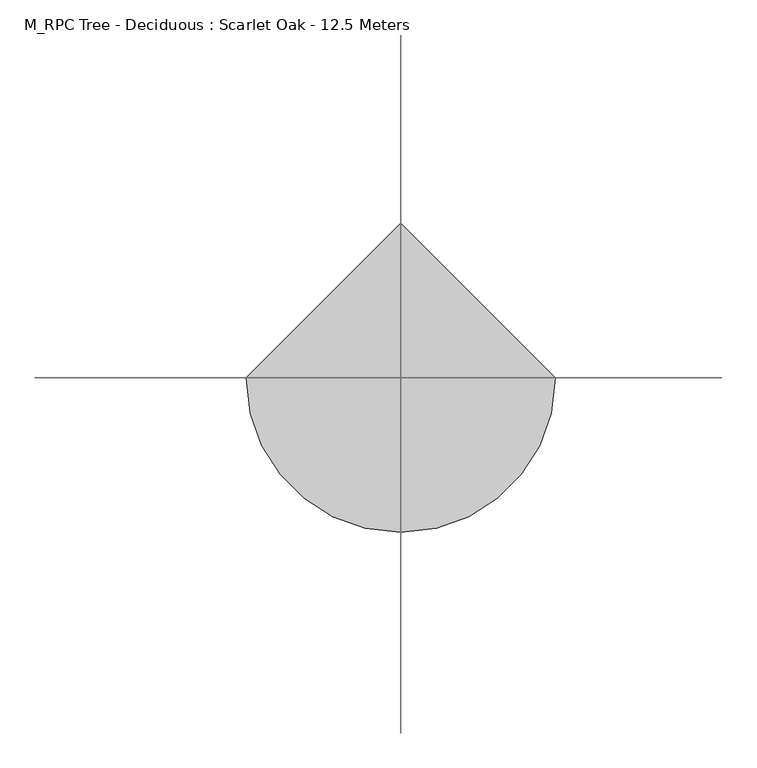
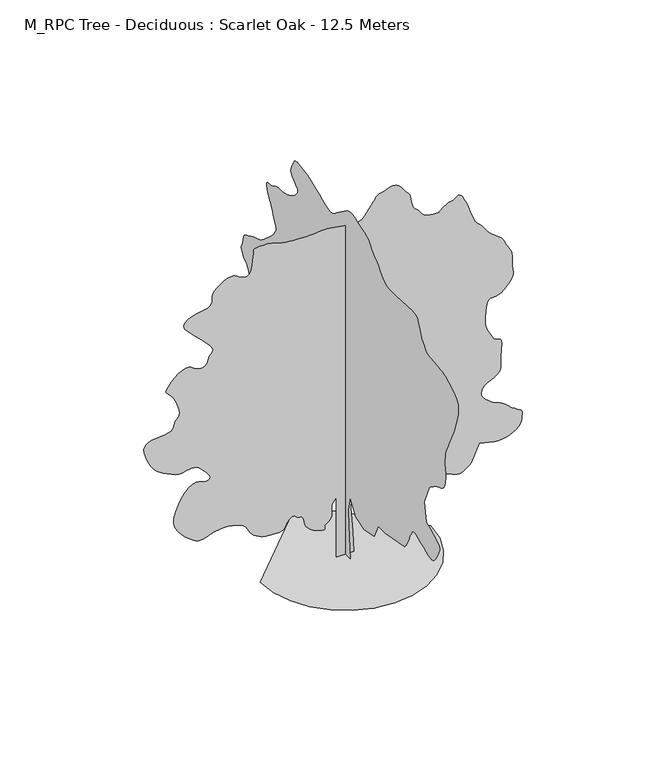
"""IFC4 building model written with IfcOpenShell, lengths in millimetres: geographic element geometry, M_RPC Tree - Deciduous : Scarlet Oak - 12.5 Meters."""

from ifc_helpers import new_model, si_unit, origin, place, context, project, spatial, triangles, source, transform, mapped, element, save


def m_rpc_tree_deciduous_scarlet_oak_12_5_meters_78a4568a(model_context):
    return source(origin(), model_context, "Body", "Tessellation", [
        triangles([(0.0172504, 306.0074844, 0.0), (0.0172504, -293.5650026, 0.0), (0.0172504, -196.8600042, 1141.1200275), (0.0172504, -177.5185068, 1682.6674953), (0.0172504, -293.5650026, 2185.5350567), (0.0172504, -603.0224945, 1682.6674953), (0.0172504, -1105.8875124, 1527.9400211), (0.0172504, -1686.1174301, 1663.3275421), (0.0172504, -1918.2099495, 2146.8525341), (0.0172504, -2324.3725124, 2146.8525341), (0.0172504, -3446.150116, 2359.6049549), (0.0172504, -3487.4249222, 2409.394939), (0.0172504, -3527.7000801, 2459.5225479), (0.0172504, -3565.9250725, 2510.3249702), (0.0172504, -3601.0999603, 2562.1500046), (0.0172504, -3632.2250954, 2615.3249565), (0.0172504, -3658.2749588, 2670.2000954), (0.0172504, -3678.2499023, 2727.0751122), (0.0172504, -3697.649881, 2785.6750237), (0.0172504, -3722.1251312, 2845.2748741), (0.0172504, -3750.8251236, 2905.7249634), (0.0172504, -3782.89991, 2966.8500114), (0.0172504, -3817.5251221, 3028.475029), (0.0172504, -3853.8249413, 3090.4500252), (0.0172504, -3890.9999977, 3152.5750122), (0.0172504, -3908.7000801, 3172.6499496), (0.0172504, -3933.1750397, 3188.8501236), (0.0172504, -3971.1750458, 3197.2499016), (0.0172504, -4029.4749756, 3193.9751015), (0.0172504, -4114.8499969, 3175.1500877), (0.0172504, -4234.0499886, 3136.8500999), (0.0172504, -4393.8501183, 3075.2250824), (0.0172504, -4562.5749939, 3002.6998581), (0.0172504, -4706.2499451, 2937.9750298), (0.0172504, -4828.2750549, 2886.4249786), (0.0172504, -4932.0251175, 2853.4999535), (0.0172504, -5020.8999252, 2844.5999153), (0.0172504, -5098.249855, 2865.125116), (0.0172504, -5167.5002792, 2920.4999336), (0.0172504, -5237.3750839, 3007.7251328), (0.0172504, -5309.5997452, 3113.9000473), (0.0172504, -5377.1002762, 3229.5499649), (0.0172504, -5432.7497864, 3345.1998825), (0.0172504, -5469.4498718, 3451.3750877), (0.0172504, -5480.1248016, 3538.6249947), (0.0172504, -5457.6250122, 3597.424894), (0.0172504, -5402.6498795, 3641.7000984), (0.0172504, -5323.3000717, 3691.0249947), (0.0172504, -5223.6747574, 3744.5999222), (0.0172504, -5107.774855, 3801.5499344), (0.0172504, -4979.7251129, 3861.0500816), (0.0172504, -4843.5499947, 3922.2251266), (0.0172504, -4703.3251236, 3984.2501198), (0.0172504, -4587.2749397, 4641.8500969), (0.0172504, -4877.3749649, 5318.7747665), (0.0172504, -4886.5249878, 5331.7001404), (0.0172504, -4900.7252838, 5347.4747589), (0.0172504, -4925.0999588, 5369.0251877), (0.0172504, -4964.6748688, 5399.20009), (0.0172504, -5024.5502838, 5440.8498734), (0.0172504, -5109.8247299, 5496.8999405), (0.0172504, -5225.5252258, 5570.225116), (0.0172504, -5351.0501221, 5636.6501312), (0.0172504, -5462.3497238, 5680.0498077), (0.0172504, -5559.4501923, 5715.3499786), (0.0172504, -5642.3497833, 5757.424736), (0.0172504, -5711.0252426, 5821.1499161), (0.0172504, -5765.4998245, 5921.4001923), (0.0172504, -5805.7502747, 6073.0752365), (0.0172504, -5829.0500153, 6222.0498642), (0.0172504, -5835.7501877, 6317.5748474), (0.0172504, -5830.6249191, 6379.6001312), (0.0172504, -5818.3750854, 6428.1000778), (0.0172504, -5803.7748138, 6483.0252136), (0.0172504, -5791.5499786, 6564.3249023), (0.0172504, -5786.4247101, 6692.0002487), (0.0172504, -5788.2251816, 6832.849791), (0.0172504, -5796.1252808, 6949.6752182), (0.0172504, -5813.8247818, 7056.3751007), (0.0172504, -5845.0502014, 7166.7747574), (0.0172504, -5893.550148, 7294.7750839), (0.0172504, -5963.0249771, 7454.2502335), (0.0172504, -6057.1750443, 7659.049942), (0.0172504, -6146.5748199, 7844.1752701), (0.0172504, -6206.1752518, 7955.8748474), (0.0172504, -6246.4751175, 8024.9502823), (0.0172504, -6277.9999374, 8082.1752777), (0.0172504, -6311.225235, 8158.3502792), (0.0172504, -6356.599791, 8284.2751511), (0.0172504, -6424.6752869, 8490.6997604), (0.0172504, -6498.0248795, 8729.4997192), (0.0172504, -6547.3747742, 8935.1499573), (0.0172504, -6565.2498459, 9112.3751862), (0.0172504, -6544.199968, 9265.925116), (0.0172504, -6476.8250107, 9400.5250397), (0.0172504, -6355.6498489, 9520.9002502), (0.0172504, -6173.2249374, 9631.8248749), (0.0172504, -5996.2252762, 9723.0001236), (0.0172504, -5879.7998245, 9785.7747803), (0.0172504, -5799.2250916, 9827.2001587), (0.0172504, -5729.8002594, 9854.4496582), (0.0172504, -5646.85009, 9874.575174), (0.0172504, -5525.6749283, 9894.699527), (0.0172504, -5341.575119, 9921.9501892), (0.0172504, -5144.0999634, 9943.4244598), (0.0172504, -4990.9500092, 9951.725116), (0.0172504, -4869.5998581, 9962.0244873), (0.0172504, -4767.5499825, 9989.5995483), (0.0172504, -4672.2499855, 10049.6505341), (0.0172504, -4571.2000488, 10157.425351), (0.0172504, -4451.8750648, 10328.0998169), (0.0172504, -4347.6750298, 10515.7499908), (0.0172504, -4286.1000092, 10666.5500885), (0.0172504, -4245.8501404, 10783.8254883), (0.0172504, -4205.5749825, 10871.0003998), (0.0172504, -4143.9999619, 10931.4501984), (0.0172504, -4039.7999268, 10968.5502594), (0.0172504, -3871.650016, 10985.7003754), (0.0172504, -2943.2749969, 10927.6748474), (0.0172504, -2772.1499771, 10930.6746643), (0.0172504, -2632.8250511, 10930.2746887), (0.0172504, -2514.4500092, 10937.3254211), (0.0172504, -2406.244986, 10962.6250397), (0.0172504, -2297.3600624, 11017.0496246), (0.0172504, -2176.9724979, 11111.3752625), (0.0172504, -2034.2550465, 11256.4745453), (0.0172504, -1896.7275398, 11403.0249023), (0.0172504, -1793.7050491, 11502.8746216), (0.0172504, -1717.0749882, 11568.5752625), (0.0172504, -1658.7125622, 11612.6248993), (0.0172504, -1610.5025688, 11647.5250946), (0.0172504, -1564.320068, 11685.7995026), (0.0172504, -1512.0500027, 11739.9996826), (0.0172504, -1461.8649845, 11804.0004272), (0.0172504, -1420.8125484, 11863.6002777), (0.0172504, -1379.087479, 11919.1503754), (0.0172504, -1326.8724976, 11970.9495392), (0.0172504, -1254.3574471, 12019.4000702), (0.0172504, -1151.7299904, 12064.7996246), (0.0172504, -1009.182514, 12107.4749268), (0.0172504, -849.1549999, 12154.4999634), (0.0172504, -699.9524792, 12206.6002716), (0.0172504, -560.5600064, 12254.6496643), (0.0172504, -429.9675053, 12289.4998627), (0.0172504, -307.1550161, 12302.0246796), (0.0172504, -191.1079934, 12283.0746735), (0.0172504, -80.8134993, 12223.5248199), (0.0172504, 499.4175176, 11798.0252106), (0.0172504, 562.2325061, 11740.8496307), (0.0172504, 623.0199657, 11688.7504852), (0.0172504, 689.217524, 11646.7751404), (0.0172504, 768.2749804, 11620.0500275), (0.0172504, 867.630035, 11613.6248383), (0.0172504, 994.7275097, 11632.5748444), (0.0172504, 1157.0125168, 11681.9753174), (0.0172504, 1341.1749676, 11755.3254913), (0.0172504, 1526.6899521, 11837.8251068), (0.0172504, 1710.1749733, 11922.0246185), (0.0172504, 1888.2475342, 12000.4500641), (0.0172504, 2057.5249924, 12065.6995697), (0.0172504, 2214.6200546, 12110.3003357), (0.0172504, 2356.1550201, 12126.8249084), (0.0172504, 2484.8875694, 12135.849939), (0.0172504, 2604.4750374, 12156.3754303), (0.0172504, 2712.9251038, 12178.575238), (0.0172504, 2808.1501053, 12192.6755402), (0.0172504, 2888.1748718, 12188.8501923), (0.0172504, 2950.9251114, 12157.2753754), (0.0172504, 2994.400074, 12088.1249451), (0.0172504, 3033.2500282, 12001.2500153), (0.0172504, 3077.8499222, 11921.1246735), (0.0172504, 3119.7499809, 11845.0502472), (0.0172504, 3150.5001389, 11770.3245758), (0.0172504, 3161.6000427, 11694.2745667), (0.0172504, 3144.6249161, 11614.1503876), (0.0172504, 3091.124984, 11527.2498779), (0.0172504, 3009.2500397, 11447.6245056), (0.0172504, 2921.5998665, 11385.2504059), (0.0172504, 2841.4251091, 11331.3502075), (0.0172504, 2781.8749649, 11277.1000305), (0.0172504, 2756.1750801, 11213.7248291), (0.0172504, 2777.4749428, 11132.4251404), (0.0172504, 2859.0249069, 11024.3747589), (0.0172504, 2971.6250107, 10916.7255157), (0.0172504, 3077.7999252, 10838.2000763), (0.0172504, 3178.2249001, 10782.3), (0.0172504, 3273.574894, 10742.6745117), (0.0172504, 3364.5248657, 10712.8251709), (0.0172504, 3451.7750633, 10686.4000397), (0.0172504, 3535.9498672, 10656.8995148), (0.0172504, 3620.024968, 10634.1753204), (0.0172504, 3706.4749237, 10626.6746155), (0.0172504, 3795.2750267, 10625.9502411), (0.0172504, 3886.4499847, 10623.5248077), (0.0172504, 3980.0000885, 10610.9499939), (0.0172504, 4075.9250473, 10579.7495728), (0.0172504, 4174.1998627, 10521.5252197), (0.0172504, 4275.775058, 10469.80047), (0.0172504, 4375.6250679, 10451.2504395), (0.0172504, 4465.0001358, 10446.8995422), (0.0172504, 4535.0999268, 10437.8245148), (0.0172504, 4577.0999794, 10405.075351), (0.0172504, 4582.2249573, 10329.6753021), (0.0172504, 4541.7001053, 10192.7255219), (0.0172504, 4481.7999825, 10048.5994354), (0.0172504, 4432.0751106, 9951.4995483), (0.0172504, 4388.424868, 9882.1247131), (0.0172504, 4346.8250816, 9821.224942), (0.0172504, 4303.1751297, 9749.5002502), (0.0172504, 4253.4249687, 9647.6750702), (0.0172504, 4193.550135, 9496.4499985), (0.0172504, 4130.2749275, 9347.6997757), (0.0172504, 4075.8250534, 9253.7502777), (0.0172504, 4034.1999779, 9195.999733), (0.0172504, 4009.500032, 9155.8498581), (0.0172504, 4005.7749687, 9114.7000443), (0.0172504, 4027.1001205, 9053.900267), (0.0172504, 4077.4999512, 8954.8999146), (0.0172504, 4167.2249977, 8823.6747849), (0.0172504, 4293.1248711, 8684.3501495), (0.0172504, 4439.3499573, 8545.349913), (0.0172504, 4589.9500671, 8415.1497208), (0.0172504, 4729.0750053, 8302.2002197), (0.0172504, 4840.7748734, 8214.9747299), (0.0172504, 4909.1747681, 8161.9000626), (0.0172504, 4969.9001312, 8128.6997635), (0.0172504, 5061.0747986, 8095.1500671), (0.0172504, 5170.5250946, 8060.9248306), (0.0172504, 5286.0750183, 8025.675238), (0.0172504, 5395.524733, 7989.0751465), (0.0172504, 5486.6999817, 7950.8001572), (0.0172504, 5547.4247635, 7910.4747116), (0.0172504, 5598.275148, 7876.9750122), (0.0172504, 5663.0252655, 7853.2997131), (0.0172504, 5734.1749924, 7830.2999542), (0.0172504, 5804.3247803, 7798.8251312), (0.0172504, 5866.0250839, 7749.7752182), (0.0172504, 5911.8001968, 7673.9751938), (0.0172504, 5934.2499893, 7562.325032), (0.0172504, 5952.6250305, 7450.1749008), (0.0172504, 5984.1998474, 7370.8500916), (0.0172504, 6018.4750809, 7312.1501862), (0.0172504, 6045.000206, 7261.899765), (0.0172504, 6053.2252853, 7207.9501511), (0.0172504, 6032.699794, 7138.074765), (0.0172504, 5972.9249542, 7040.1249298), (0.0172504, 5898.7248322, 6948.3747162), (0.0172504, 5838.7250061, 6893.5251572), (0.0172504, 5788.2001831, 6857.9500031), (0.0172504, 5742.4000717, 6824.0497467), (0.0172504, 5696.6249588, 6774.2498795), (0.0172504, 5646.1001358, 6690.9747299), (0.0172504, 5586.0997284, 6556.5997925), (0.0172504, 5520.7002319, 6421.9998688), (0.0172504, 5460.6998245, 6337.1498154), (0.0172504, 5411.5249191, 6283.075209), (0.0172504, 5378.6001846, 6240.824881), (0.0172504, 5367.3247101, 6191.4999847), (0.0172504, 5383.09991, 6116.0999359), (0.0172504, 5431.3748703, 5995.7247253), (0.0172504, 5495.5000259, 5864.0502045), (0.0172504, 5555.8748291, 5761.8250488), (0.0172504, 5613.5747955, 5680.5747757), (0.0172504, 5669.5498672, 5611.8249023), (0.0172504, 5724.8749786, 5547.1497803), (0.0172504, 5780.5250702, 5478.0749268), (0.0172504, 5837.5250793, 5396.1502762), (0.0172504, 5903.6751114, 5315.3499756), (0.0172504, 5980.6500641, 5249.4249298), (0.0172504, 6060.324852, 5189.6000931), (0.0172504, 6134.5999695, 5127.0498413), (0.0172504, 6195.3247513, 5053.0252899), (0.0172504, 6234.4002731, 4958.675235), (0.0172504, 6243.7002869, 4835.2499199), (0.0172504, 6251.5248093, 4738.3250221), (0.0172504, 6280.349794, 4706.349939), (0.0172504, 6313.2251129, 4704.825032), (0.0172504, 6333.2500534, 4699.2500816), (0.0172504, 6323.4750687, 4655.0998695), (0.0172504, 6267.0500244, 4537.8750481), (0.0172504, 6146.999794, 4313.0501083), (0.0172504, 6021.4748978, 4060.8750938), (0.0172504, 5945.6998718, 3875.3750793), (0.0172504, 5898.3248566, 3742.6250427), (0.0172504, 5858.0749878, 3648.7999557), (0.0172504, 5803.5998245, 3580.0000854), (0.0172504, 5713.6000854, 3522.3751144), (0.0172504, 5566.7747452, 3462.0500175), (0.0172504, 5397.250209, 3413.1000984), (0.0172504, 5248.0500137, 3392.5748978), (0.0172504, 5111.025238, 3390.9999939), (0.0172504, 4978.0752136, 3398.9000931), (0.0172504, 4841.0498566, 3406.7749031), (0.0172504, 4691.8499519, 3405.1999992), (0.0172504, 4522.3501236, 3384.6750893), (0.0172504, 4353.2999771, 3366.3000481), (0.0172504, 4207.2498802, 3370.2500977), (0.0172504, 4078.7998718, 3385.7000267), (0.0172504, 3962.5249924, 3401.8249146), (0.0172504, 3853.0249901, 3407.8001312), (0.0172504, 3744.8749054, 3392.799884), (0.0172504, 3632.6500694, 3346.0001244), (0.0172504, 3525.249939, 3296.2499634), (0.0172504, 3436.4251282, 3270.2000999), (0.0172504, 3368.249929, 3253.6249489), (0.0172504, 3322.75009, 3232.3250862), (0.0172504, 3301.9499062, 3192.0499283), (0.0172504, 3307.8751259, 3118.6500481), (0.0172504, 3342.5500443, 2997.8498634), (0.0172504, 3398.475119, 2869.5251381), (0.0172504, 3465.5750931, 2778.7248665), (0.0172504, 3542.0000793, 2719.2500084), (0.0172504, 3625.8499031, 2684.8000763), (0.0172504, 3715.274968, 2669.1248703), (0.0172504, 3808.4250961, 2665.9500641), (0.0172504, 3903.4251114, 2669.0498749), (0.0172504, 4270.9250633, 2262.8999565), (0.0172504, 4299.7250496, 2217.1674282), (0.0172504, 4327.3501076, 2170.5925095), (0.0172504, 4352.6250183, 2122.3249615), (0.0172504, 4374.3248566, 2071.5174522), (0.0172504, 4391.2999832, 2017.3300621), (0.0172504, 4402.3498901, 1958.9125523), (0.0172504, 4406.2999397, 1895.4200615), (0.0172504, 4405.6249809, 1829.2200325), (0.0172504, 4400.8999786, 1763.6974331), (0.0172504, 4388.0248924, 1699.5299835), (0.0172504, 4362.9999664, 1637.3900265), (0.0172504, 4321.7248695, 1577.9574623), (0.0172504, 4260.1501396, 1521.9075405), (0.0172504, 4174.1998627, 1469.9175453), (0.0172504, 4092.2249245, 1425.7650078), (0.0172504, 4034.5999535, 1391.4249527), (0.0172504, 3985.4250481, 1364.8675621), (0.0172504, 3928.800016, 1344.0599659), (0.0172504, 3848.8499542, 1326.9749622), (0.0172504, 3729.6499626, 1311.5799717), (0.0172504, 3555.3001396, 1295.8475018), (0.0172504, 3356.9750359, 1298.1024513), (0.0172504, 3174.2251442, 1332.8375404), (0.0172504, 3003.6500908, 1392.27243), (0.0172504, 2841.8750816, 1468.6199501), (0.0172504, 2685.525032, 1554.1049938), (0.0172504, 2531.1748604, 1640.9425713), (0.0172504, 2375.4949734, 1721.3500179), (0.0172504, 2236.6675461, 1794.4849434), (0.0172504, 2129.3050587, 1863.5599422), (0.0172504, 2044.6099377, 1926.8850014), (0.0172504, 1973.7875164, 1982.7650208), (0.0172504, 1908.0399307, 2029.5099873), (0.0172504, 1838.5700432, 2065.4300331), (0.0172504, 1756.5824604, 2088.8300583), (0.0172504, 1666.4174698, 2108.5650455), (0.0172504, 1577.6074837, 2133.0375343), (0.0172504, 1489.134977, 2159.8799366), (0.0172504, 1399.9875114, 2186.7200134), (0.0172504, 1309.1449459, 2211.1925022), (0.0172504, 1215.5975309, 2230.9274895), (0.0172504, 1118.3299942, 2243.5575325), (0.0172504, 1018.8625191, 2250.1549496), (0.0172504, 919.3925005, 2253.7074944), (0.0172504, 819.9250254, 2254.7225487), (0.0172504, 720.4574776, 2253.7074944), (0.0172504, 620.9900024, 2251.1700039), (0.0172504, 521.5199839, 2247.6174591), (0.0172504, 422.0525087, 2243.5575325), (0.0172504, 228.6430025, 1953.4425373), (0.0172504, 189.960498, 1508.6000679), (280.4450004, 0.0006008, 0.0092122), (-299.7850081, 0.0006008, 0.0092122), (-299.7850081, 0.0004756, 2127.5199932), (-454.5149895, 0.0004756, 1914.7700432), (-454.5149895, 0.0005007, 1682.6775238), (-450.9625174, 0.0005007, 1628.8274677), (-450.9625174, 0.0005007, 1575.1449886), (-458.0674979, 0.0005007, 1521.8024597), (-475.8274967, 0.0005257, 1468.967458), (-507.8000001, 0.0005257, 1416.8100311), (-557.5350094, 0.0005257, 1365.4949947), (-628.5824896, 0.0005257, 1315.1974834), (-684.2375227, 0.0005257, 1262.982502), (-699.6325132, 0.0005257, 1210.0900183), (-696.0799685, 0.0005257, 1162.9524885), (-694.8950117, 0.0005257, 1127.990015), (-717.3950191, 0.0005257, 1111.6375248), (-784.8900272, 0.0005257, 1120.3225325), (-918.6974848, 0.0005257, 1160.4700092), (-1071.3399845, 0.0005257, 1223.0050003), (-1185.4125275, 0.0005257, 1293.6575191), (-1267.3425556, 0.0005257, 1371.0799736), (-1323.5625252, 0.0005257, 1453.9125629), (-1360.49748, 0.0005007, 1540.8049335), (-1384.5749348, 0.0005007, 1630.4049877), (-1402.2250202, 0.0005007, 1721.3600464), (-1406.7350647, 0.0005007, 1746.1124599), (-1413.4449749, 0.0005007, 1770.19006), (-1424.5524364, 0.0005007, 1792.9174519), (-1442.2599312, 0.0005007, 1813.6099388), (-1468.7600578, 0.0005007, 1831.5975037), (-1506.2599491, 0.0005007, 1846.2025715), (-1556.9524944, 0.0005007, 1856.7475674), (-1607.6450397, 0.0005007, 1874.1124958), (-1647.5100483, 0.0005007, 1903.3224861), (-1682.3025467, 0.0004756, 1934.9000645), (-1717.7700039, 0.0004756, 1959.3725533), (-1759.6674465, 0.0004756, 1967.2675655), (-1813.7424889, 0.0004756, 1949.1099529), (-1885.7500122, 0.0005007, 1895.4274738), (-1949.0724552, 0.0005007, 1820.3199944), (-1984.9925011, 0.0005007, 1746.902528), (-2011.1000645, 0.0005007, 1679.2374722), (-2044.9875309, 0.0005007, 1621.382428), (-2104.2525181, 0.0005007, 1577.4025543), (-2206.4824699, 0.0005007, 1551.3499294), (-2369.2750042, 0.0005007, 1547.2900028), (-2549.149926, 0.0005007, 1559.2449417), (-2695.2000229, 0.0005007, 1578.979929), (-2813.8250496, 0.0005007, 1607.1750103), (-2911.4999016, 0.0005007, 1644.5025284), (-2994.6250603, 0.0005007, 1691.6425289), (-3069.600135, 0.0005007, 1749.2724415), (-3142.9250198, 0.0005007, 1818.0650448), (-3205.1000038, 0.0005007, 1893.5100037), (-3249.7248962, 0.0004756, 1969.2975288), (-3287.549913, 0.0004756, 2043.389954), (-3329.4499718, 0.0004756, 2113.7625481), (-3386.2249947, 0.0004756, 2178.3824409), (-3468.7249008, 0.0004756, 2235.2224308), (-3587.7499031, 0.0004756, 2282.2499382), (-3707.4248657, 0.0004756, 2317.9974655), (-3794.2500893, 0.0004506, 2343.2600224), (-3862.8249733, 0.0004506, 2359.3875263), (-3927.6750847, 0.0004506, 2367.7325111), (-4003.3251183, 0.0004506, 2369.6499813), (-4104.3750549, 0.0004506, 2366.4924706), (-4245.3498802, 0.0004506, 2359.6125126), (-4400.3500122, 0.0004506, 2335.1974331), (-4538.1250328, 0.0004756, 2289.8050003), (-4665.0501343, 0.0004756, 2240.3524956), (-4787.5749229, 0.0004756, 2203.7574909), (-4912.1501678, 0.0004756, 2196.9349422), (-5045.1501892, 0.0004756, 2236.7999508), (-5193.0498825, 0.0004506, 2340.2725594), (-5347.7997391, 0.0004506, 2478.6475433), (-5490.6747391, 0.0004506, 2615.9999153), (-5612.2498764, 0.0004256, 2758.4499413), (-5703.0251495, 0.0004256, 2912.049868), (-5753.5499725, 0.0004256, 3082.8999046), (-5754.3499237, 0.0004005, 3277.0999695), (-5695.9250015, 0.0004005, 3500.7249825), (-5598.1501556, 0.0003755, 3726.2748779), (-5489.1998291, 0.0003755, 3919.6999901), (-5372.1499969, 0.0003505, 4077.2499664), (-5250.0248932, 0.0003505, 4195.2000343), (-5125.8499146, 0.0003505, 4269.8501289), (-5002.6998734, 0.0003505, 4297.4998947), (-4883.6001663, 0.0003505, 4274.3751434), (-4771.2750458, 0.0003505, 4235.4749016), (-4671.8250114, 0.0003505, 4218.8750427), (-4593.3248611, 0.0003505, 4225.6499199), (-4543.9249695, 0.0003505, 4256.7750549), (-4531.7501312, 0.0003505, 4313.2750946), (-4564.9001427, 0.0003505, 4396.1749763), (-4651.5000893, 0.0003254, 4506.4749298), (-4752.500029, 0.0003254, 4617.0998634), (-4829.4749817, 0.0003254, 4702.3498924), (-4891.5502625, 0.0003254, 4765.2751213), (-4947.8747314, 0.0003254, 4808.9250732), (-5007.6001556, 0.0003254, 4836.325145), (-5079.8248169, 0.0003004, 4850.5498581), (-5173.7248993, 0.0003004, 4854.5999016), (-5270.0248352, 0.0003254, 4845.5248741), (-5349.7751999, 0.0003254, 4824.5999886), (-5422.3998367, 0.0003254, 4801.3249557), (-5497.39991, 0.0003254, 4785.1250725), (-5584.2248428, 0.0003254, 4785.5250481), (-5692.3752182, 0.0003254, 4811.9748871), (-5831.3248764, 0.0003004, 4873.9498833), (-5978.7751785, 0.0003004, 4948.0997177), (-6108.6248108, 0.0003004, 5012.4248611), (-6224.6252884, 0.0003004, 5078.4748993), (-6330.4502243, 0.0003004, 5157.6997147), (-6429.8749695, 0.0003004, 5261.5997681), (-6526.574881, 0.0002754, 5401.7249359), (-6624.2997299, 0.0002754, 5589.5750977), (-6705.1000305, 0.0002503, 5784.4998276), (-6749.7002151, 0.0002503, 5941.2001465), (-6759.8001801, 0.0002503, 6064.0752045), (-6737.074823, 0.0002253, 6157.4997345), (-6683.2252029, 0.0002253, 6225.9002106), (-6599.9500534, 0.0002253, 6273.6502029), (-6488.899855, 0.0002253, 6305.1750229), (-6357.7997177, 0.0002253, 6323.2750809), (-6219.2750336, 0.0002253, 6333.9500107), (-6082.4002487, 0.0002253, 6346.2748398), (-5956.3748016, 0.0002253, 6369.4501694), (-5850.3248795, 0.0002253, 6412.5998611), (-5773.3499268, 0.0002253, 6484.8251038), (-5734.5999664, 0.0002003, 6595.2997559), (-5705.9749695, 0.0002003, 6701.9752213), (-5661.749762, 0.0002003, 6771.4500504), (-5614.8497177, 0.0002003, 6825.7002274), (-5578.0752182, 0.0002003, 6886.6999924), (-5564.3248947, 0.0001752, 6976.4747452), (-5586.4252899, 0.0001752, 7116.9998886), (-5657.2500366, 0.0001752, 7330.2502441), (-5757.5497284, 0.0001502, 7540.3002136), (-5853.4752686, 0.0001502, 7672.5252823), (-5935.8498917, 0.0001502, 7750.975145), (-5995.5747345, 0.0001252, 7799.6250824), (-6023.4747757, 0.0001252, 7842.5247894), (-6010.4499893, 0.0001252, 7903.7251236), (-5947.3497711, 0.0001252, 8007.2002029), (-5845.6501648, 0.0001252, 8136.3248795), (-5728.0247864, 0.0001001, 8253.9502579), (-5602.2749039, 0.0001001, 8353.3000076), (-5476.1750427, 0.0001001, 8427.6251221), (-5357.5497253, 0.0001001, 8470.1248535), (-5254.1252243, 0.0001001, 8474.0751938), (-5173.7248993, 0.0001001, 8432.6998123), (-5094.9000595, 0.0001001, 8371.00009), (-4997.8001724, 0.0001001, 8322.8501221), (-4892.5751999, 0.0001001, 8294.6500992), (-4789.3751038, 0.0001001, 8292.850209), (-4698.375135, 0.0001001, 8323.8750595), (-4629.6999664, 0.0001001, 8394.1248413), (-4593.5001411, 0.0001001, 8510.0497421), (-4560.3251312, 0.0001001, 8620.5749725), (-4508.2251137, 7.51e-05, 8686.1000427), (-4458.4999512, 7.51e-05, 8730.3002518), (-4432.4500877, 7.51e-05, 8776.8747345), (-4451.4000938, 7.51e-05, 8849.4999527), (-4536.6501228, 7.51e-05, 8971.8750412), (-4709.5500343, 5.01e-05, 9167.6497192), (-4926.3498825, 5.01e-05, 9388.800174), (-5120.1502625, 2.5e-05, 9575.0998489), (-5277.4249649, 2.5e-05, 9731.9751572), (-5384.5998184, 2.5e-05, 9864.8246063), (-5428.2000641, 0.0, 9979.0746094), (-5394.6497864, 0.0, 10080.1254181), (-5270.4248108, 0.0, 10173.3755402), (-5104.7500397, 0.0, 10245.2246429), (-4956.3497955, 0.0, 10286.2744629), (-4825.8749107, 0.0, 10308.3754395), (-4714.0000534, -2.5e-05, 10323.3745239), (-4621.3998917, -2.5e-05, 10343.1000641), (-4548.7749641, -2.5e-05, 10379.4245911), (-4496.7749405, -2.5e-05, 10444.1497101), (-4470.8500694, -2.5e-05, 10520.7252686), (-4466.9000198, -2.5e-05, 10587.8246613), (-4471.4000359, -2.5e-05, 10650.1999237), (-4470.8500694, -2.5e-05, 10712.5751862), (-4451.6750771, -5.01e-05, 10779.6745789), (-4400.3500122, -5.01e-05, 10856.2501373), (-4303.3751175, -5.01e-05, 10947.0248291), (-4184.6750954, -5.01e-05, 11036.8495789), (-4076.1250351, -5.01e-05, 11106.7255463), (-3976.0500389, -7.51e-05, 11155.60047), (-3882.7249214, -7.51e-05, 11182.4999908), (-3794.4750755, -7.51e-05, 11186.3997528), (-3709.6000237, -7.51e-05, 11166.2498199), (-3626.4498665, -5.01e-05, 11121.1002502), (-3540.7248665, -5.01e-05, 11065.9001312), (-3452.3250298, -5.01e-05, 11022.8748505), (-3365.6000908, -5.01e-05, 11001.8249725), (-3284.9500717, -5.01e-05, 11012.5998962), (-3214.7999931, -5.01e-05, 11064.9746063), (-3159.5498772, -7.51e-05, 11168.7996643), (-3123.5750381, -7.51e-05, 11333.8500549), (-3102.0998955, -7.51e-05, 11511.0752838), (-3086.6999634, -0.0001001, 11648.0250641), (-3076.3750122, -0.0001001, 11749.4746857), (-3070.125103, -0.0001001, 11820.1250244), (-3066.9000092, -0.0001001, 11864.7246277), (-3065.7250809, -0.0001001, 11888.025531), (-3065.5500916, -0.0001001, 11894.7251221), (-3040.1248993, -0.0001001, 11898.674881), (-2971.0500458, -0.0001001, 11907.3755127), (-2869.1498703, -0.0001001, 11916.0505646), (-2745.2748734, -0.0001001, 11920.0003235), (-2610.2249771, -0.0001001, 11914.4750793), (-2474.8323692, -0.0001001, 11894.7251221), (-2349.935051, -0.0001001, 11856.0495758), (-2235.4100647, -0.0001001, 11813.0254578), (-2120.5474537, -0.0001001, 11781.8494537), (-2000.2725277, -0.0001001, 11760.1251984), (-1869.5075443, -0.0001001, 11745.5249268), (-1723.1824642, -0.0001001, 11735.675528), (-1556.2175102, -0.0001001, 11728.174823), (-1363.5400269, -0.0001001, 11720.6752808), (-1177.5749971, -0.0001001, 11719.599765), (-1024.4249702, -0.0001001, 11728.6747925), (-889.5449764, -0.0001001, 11741.475174), (-758.3875025, -0.0001001, 11751.5745575), (-616.4050352, -0.0001001, 11752.5244995), (-449.0450109, -0.0001001, 11737.9253906), (-241.763259, -0.0001001, 11701.3252991), (-32.2257492, -0.0001001, 11657.8000488), (136.7125037, -0.0001001, 11627.7995544), (271.8174929, -0.0001001, 11613.0248749), (379.8574825, -0.0001001, 11615.1503265), (467.5975121, -0.0001001, 11635.9246399), (541.8025031, -0.0001001, 11676.9744598), (609.2425, -0.0001001, 11739.9996826), (899.3575315, -0.0001252, 12107.4749268), (942.8899761, -0.0001252, 12164.1505371), (977.6249926, -0.0001252, 12217.4496094), (1008.9749685, -0.0001252, 12266.3245331), (1042.3575239, -0.0001252, 12309.7997864), (1083.1825029, -0.0001252, 12346.8498505), (1136.864982, -0.0001252, 12376.4503693), (1208.8150234, -0.0001252, 12397.6002411), (1297.0049892, -0.0001502, 12421.8499237), (1393.3149536, -0.0001502, 12454.2246918), (1494.0224693, -0.0001502, 12483.8752075), (1595.4100307, -0.0001502, 12499.9998047), (1693.7499584, -0.0001502, 12491.7747253), (1785.3225666, -0.0001502, 12448.349469), (1866.410059, -0.0001252, 12358.9246948), (1938.4149662, -0.0001252, 12256.9251068), (2004.3324543, -0.0001252, 12177.5752991), (2062.8075188, -0.0001252, 12112.7746033), (2112.4850098, -0.0001252, 12054.4246765), (2152.0125389, -0.0001252, 11994.3748535), (2180.0375725, -0.0001001, 11924.5000488), (2195.2049606, -0.0001001, 11836.6995941), (2205.7499565, -0.0001001, 11745.7004974), (2220.3550243, -0.0001001, 11669.9248901), (2238.3424438, -0.0001001, 11606.8252533), (2259.0349308, -7.51e-05, 11553.8749969), (2281.7599972, -7.51e-05, 11508.5254395), (2305.8374519, -7.51e-05, 11468.2755707), (2330.5924816, -7.51e-05, 11430.5499664), (2355.6274361, -7.51e-05, 11413.5754211), (2381.680061, -7.51e-05, 11394.2254395), (2409.760033, -7.51e-05, 11370.1501648), (2440.8876389, -7.51e-05, 11338.9753235), (2476.0724098, -7.51e-05, 11298.3254791), (2516.3248947, -7.51e-05, 11245.8251953), (2562.6749725, -7.51e-05, 11179.1246155), (2631.3751396, -5.01e-05, 11115.7249969), (2728.4750267, -5.01e-05, 11072.3253204), (2839.7749191, -5.01e-05, 11045.1246552), (2951.0751022, -5.01e-05, 11030.4755493), (3048.1749893, -5.01e-05, 11024.6003265), (3116.8748657, -5.01e-05, 11023.8247925), (3142.9250198, -5.01e-05, 11024.4003387), (3156.2750771, -5.01e-05, 11038.3250702), (3192.9998703, -5.01e-05, 11074.2252045), (3247.9750031, -5.01e-05, 11123.3501129), (3316.1499115, -7.51e-05, 11176.8503357), (3392.4249069, -7.51e-05, 11225.9752441), (3471.7750053, -7.51e-05, 11261.8997955), (3549.0749382, -7.51e-05, 11275.824527), (3618.3750687, -7.51e-05, 11292.800235), (3679.5501137, -7.51e-05, 11331.0746429), (3736.350135, -7.51e-05, 11371.7244873), (3792.4499084, -7.51e-05, 11395.8253418), (3851.6000771, -7.51e-05, 11384.3748779), (3917.5251228, -7.51e-05, 11318.4498322), (3993.9251106, -7.51e-05, 11179.1246155), (4065.8750793, -5.01e-05, 11015.4253052), (4119.5500008, -5.01e-05, 10883.1996552), (4160.3751251, -5.01e-05, 10773.6249481), (4193.7501228, -2.5e-05, 10677.9505554), (4225.0999535, -2.5e-05, 10587.3246918), (4259.8498672, -2.5e-05, 10493.0002167), (4303.3751175, -2.5e-05, 10386.1253448), (4348.1000038, 0.0, 10292.3496735), (4386.3749931, 0.0, 10232.749823), (4423.6500435, 0.0, 10191.7755798), (4465.325116, 0.0, 10153.8255707), (4516.799881, 0.0, 10103.3495819), (4583.4998795, 0.0, 10024.7997253), (4670.850071, 0.0, 9902.6002075), (4778.3749031, 2.5e-05, 9766.6003693), (4896.3999664, 2.5e-05, 9652.9247498), (5016.4501968, 2.5e-05, 9555.474884), (5130.075238, 5.01e-05, 9468.1999786), (5228.8000259, 5.01e-05, 9384.974826), (5304.2000748, 5.01e-05, 9299.6997986), (5347.7997391, 5.01e-05, 9206.3252655), (5382.0249756, 5.01e-05, 9114.7500412), (5429.774968, 7.51e-05, 9032.6498199), (5483.3001892, 7.51e-05, 8950.5501801), (5534.7749542, 7.51e-05, 8858.9749557), (5576.449736, 7.51e-05, 8748.4747238), (5600.5250107, 0.0001001, 8609.5250656), (5599.22509, 0.0001001, 8432.6998123), (5596.5752518, 0.0001001, 8262.7497208), (5611.174942, 0.0001252, 8138.7997284), (5627.1251312, 0.0001252, 8042.949765), (5628.5500443, 0.0001252, 7957.224765), (5599.5000732, 0.0001252, 7863.750238), (5524.1250229, 0.0001502, 7744.5249573), (5386.4752853, 0.0001502, 7581.6750137), (5223.124791, 0.0001502, 7444.9502197), (5081.4247192, 0.0001502, 7390.0750809), (4961.7000504, 0.0001502, 7378.1752258), (4864.3248894, 0.0001502, 7370.3501221), (4789.60009, 0.0001752, 7327.6498215), (4737.9000481, 0.0001752, 7211.2249512), (4709.5250359, 0.0001752, 6982.1249817), (4698.9251015, 0.0002003, 6728.5997589), (4700.5250038, 0.0002003, 6550.1751846), (4714.6000168, 0.0002253, 6424.9002731), (4741.5751144, 0.0002253, 6330.7252075), (4781.7249893, 0.0002253, 6245.7001648), (4835.3999107, 0.0002253, 6147.7997452), (4902.950148, 0.0002503, 6015.0752884), (4980.0250946, 0.0002503, 5899.6497757), (5057.7999985, 0.0002503, 5847.1500732), (5129.8002548, 0.0002503, 5825.7752151), (5189.6250916, 0.0002503, 5803.7248169), (5230.8499008, 0.0002503, 5749.200238), (5247.0250763, 0.0002754, 5630.3749329), (5231.7498459, 0.0002754, 5415.5002579), (5210.9999496, 0.0003004, 5178.6001831), (5207.8251434, 0.0003004, 5005.3247131), (5211.4499222, 0.0003004, 4881.0997375), (5210.9999496, 0.0003254, 4791.3999802), (5195.6497238, 0.0003254, 4721.6498772), (5154.5999039, 0.0003254, 4657.3000259), (5077.0249878, 0.0003254, 4583.8248596), (4983.2998947, 0.0003254, 4514.9249954), (4900.3997223, 0.0003254, 4468.3499313), (4827.3251129, 0.0003254, 4435.6498924), (4763.0499664, 0.0003505, 4408.3501053), (4706.5499268, 0.0003505, 4378.0249214), (4656.8250549, 0.0003505, 4336.1748596), (4612.8251244, 0.0003505, 4274.3751434), (4577.8749321, 0.0003505, 4202.8248596), (4558.1249748, 0.0003505, 4135.32491), (4557.0000435, 0.0003505, 4068.8498978), (4577.8749321, 0.0003755, 4000.3250107), (4624.1000175, 0.0003755, 3926.7501411), (4699.1000908, 0.0003755, 3845.024897), (4806.2499458, 0.0003755, 3752.1750412), (4919.8002823, 0.0003755, 3670.8000664), (5016.1252167, 0.0003755, 3617.5001221), (5101.6002319, 0.0004005, 3580.1250778), (5182.6999329, 0.0004005, 3546.4750969), (5265.8000931, 0.0004005, 3504.3500519), (5357.374736, 0.0004005, 3441.5751045), (5463.8252151, 0.0004005, 3346.0001244), (5576.8497116, 0.0004005, 3247.2750458), (5681.0497467, 0.0004005, 3176.6249977), (5772.3999847, 0.0004256, 3124.2249985), (5846.8250931, 0.0004256, 3080.3000633), (5900.2747375, 0.0004256, 3035.0249199), (5928.6997467, 0.0004256, 2978.5748772), (5928.0247879, 0.0004256, 2901.1499519), (5916.924884, 0.0004256, 2813.2500847), (5910.1997131, 0.0004506, 2730.7498878), (5898.0748718, 0.0004506, 2651.975045), (5870.7247971, 0.0004506, 2575.2500771), (5818.350087, 0.0004506, 2498.8349739), (5731.1251785, 0.0004506, 2421.0750401), (5599.22509, 0.0004506, 2340.2725594), (5441.7248199, 0.0004756, 2274.8624531), (5284.2501297, 0.0004756, 2240.917432), (5126.7498596, 0.0004756, 2233.1924675), (4969.2501709, 0.0004756, 2246.4425308), (4811.7748993, 0.0004756, 2275.4250641), (4654.2749199, 0.0004756, 2314.8975094), (4496.7749405, 0.0004506, 2359.6125126), (4225.9998985, 0.0005007, 1760.042569), (4159.6498787, 0.0005007, 1702.5250042), (4092.9248817, 0.0005007, 1648.0549278), (4025.5499245, 0.0005007, 1599.675032), (3957.1500298, 0.0005007, 1560.4274277), (3887.3999268, 0.0005007, 1533.3625099), (3815.9499275, 0.0005007, 1521.5225349), (3742.4750519, 0.0005007, 1527.9500496), (3682.5999275, 0.0005007, 1542.5525013), (3644.6999153, 0.0005007, 1554.7899811), (3617.6501129, 0.0005007, 1567.0274609), (3590.2500412, 0.0005007, 1581.6300579), (3551.3250916, 0.0005007, 1600.9724819), (3489.750071, 0.0005007, 1627.4175247), (3394.3500801, 0.0005007, 1663.3375706), (3270.0751076, 0.0005007, 1715.4949974), (3134.2999649, 0.0005007, 1784.5699963), (2994.450071, 0.0005007, 1863.794957), (2857.9999695, 0.0004756, 1946.40256), (2732.3500809, 0.0004756, 2025.6275208), (2624.9999474, 0.0004756, 2094.7025196), (2543.3499893, 0.0004756, 2146.8625626), (2474.2126396, 0.0004756, 2192.817461), (2400.0074306, 0.0004756, 2246.8925034), (2321.5700672, 0.0004756, 2307.7374813), (2239.7525322, 0.0004506, 2373.9924488), (2155.3950359, 0.0004506, 2444.3074883), (2069.3475266, 0.0004506, 2517.3251244), (1982.4550106, 0.0004506, 2591.6999451), (1963.1124413, 0.0004256, 2881.8249687), (1576.2924477, 0.0004256, 2920.4999336), (880.0150349, 0.0004256, 2862.474987), (415.8325032, 0.0004506, 2611.0499268), (222.4215072, 0.0004756, 2146.8625626), (183.7397477, 0.0005007, 1605.3124786), (241.7622416, 0.0005507, 715.6274672), (-2855.9000977, 0.0, 0.0224297), (-2780.4000549, -654.3849844, 0.0224297), (-2565.3750984, -1255.3350037, 0.0224297), (-2228.0500488, -1785.6274899, 0.0224297), (-1785.6274899, -2228.0500488, 0.0224297), (-1255.3350037, -2565.3750984, 0.0224297), (-654.3849844, -2780.4000549, 0.0224297), (0.0001248, -2855.9000977, 0.0224297), (654.3849844, -2780.4000549, 0.0224297), (1255.3350037, -2565.3750984, 0.0224297), (1785.6274899, -2228.0500488, 0.0224297), (2228.0500488, -1785.6274899, 0.0224297), (2565.3750984, -1255.3350037, 0.0224297), (2780.4000549, -654.3849844, 0.0224297), (2855.9000977, 0.0002503, 0.0224297), (-0.0003745, 2855.9000977, 0.0224297)], [[1, 2, 3], [368, 1, 3], [368, 3, 4], [367, 368, 4], [367, 4, 5], [277, 278, 279], [366, 367, 5], [276, 277, 279], [276, 279, 280], [7, 8, 9], [6, 7, 9], [5, 6, 9], [315, 316, 317], [201, 202, 203], [200, 201, 203], [200, 203, 204], [199, 200, 204], [199, 204, 205], [198, 199, 205], [198, 205, 206], [198, 206, 207], [197, 198, 207], [197, 207, 208], [275, 276, 280], [196, 197, 208], [195, 196, 208], [194, 195, 208], [194, 208, 209], [193, 194, 209], [192, 193, 209], [192, 209, 210], [191, 192, 210], [191, 210, 211], [191, 211, 212], [190, 191, 212], [190, 212, 213], [190, 213, 214], [189, 190, 214], [189, 214, 215], [188, 189, 215], [187, 188, 215], [186, 187, 215], [10, 11, 12], [314, 315, 317], [10, 12, 13], [10, 13, 14], [10, 14, 15], [10, 15, 16], [10, 16, 17], [10, 17, 18], [10, 18, 19], [10, 19, 20], [10, 20, 21], [10, 21, 22], [185, 186, 215], [185, 215, 216], [275, 280, 281], [10, 22, 23], [167, 168, 169], [166, 167, 169], [165, 166, 169], [165, 169, 170], [164, 165, 170], [164, 170, 171], [163, 164, 171], [163, 171, 172], [163, 172, 173], [163, 173, 174], [163, 174, 175], [163, 175, 176], [163, 176, 177], [163, 177, 178], [163, 178, 179], [163, 179, 180], [162, 163, 180], [161, 162, 180], [160, 161, 180], [159, 160, 180], [159, 180, 181], [158, 159, 181], [157, 158, 181], [156, 157, 181], [156, 181, 182], [155, 156, 182], [154, 155, 182], [154, 182, 183], [9, 10, 23], [9, 23, 24], [9, 24, 25], [45, 46, 47], [44, 45, 47], [44, 47, 48], [43, 44, 48], [43, 48, 49], [42, 43, 49], [42, 49, 50], [41, 42, 50], [40, 41, 50], [40, 50, 51], [39, 40, 51], [38, 39, 51], [37, 38, 51], [36, 37, 51], [35, 36, 51], [34, 35, 51], [33, 34, 51], [33, 51, 52], [32, 33, 52], [32, 52, 53], [31, 32, 53], [30, 31, 53], [29, 30, 53], [28, 29, 53], [28, 53, 54], [27, 28, 54], [26, 27, 54], [5, 9, 25], [5, 25, 26], [5, 26, 54], [5, 54, 55], [366, 5, 55], [365, 366, 55], [364, 365, 55], [363, 364, 55], [362, 363, 55], [361, 362, 55], [361, 55, 56], [153, 154, 183], [153, 183, 184], [313, 314, 317], [360, 361, 56], [184, 185, 216], [153, 184, 216], [152, 153, 216], [152, 216, 217], [243, 244, 245], [242, 243, 245], [242, 245, 246], [241, 242, 246], [241, 246, 247], [241, 247, 248], [240, 241, 248], [240, 248, 249], [240, 249, 250], [239, 240, 250], [239, 250, 251], [238, 239, 251], [237, 238, 251], [236, 237, 251], [235, 236, 251], [234, 235, 251], [233, 234, 251], [232, 233, 251], [231, 232, 251], [230, 231, 251], [229, 230, 251], [228, 229, 251], [228, 251, 252], [227, 228, 252], [226, 227, 252], [226, 252, 253], [226, 253, 254], [226, 254, 255], [226, 255, 256], [226, 256, 257], [225, 226, 257], [224, 225, 257], [223, 224, 257], [222, 223, 257], [222, 257, 258], [221, 222, 258], [220, 221, 258], [115, 116, 117], [114, 115, 117], [114, 117, 118], [113, 114, 118], [113, 118, 119], [112, 113, 119], [111, 112, 119], [110, 111, 119], [152, 217, 218], [313, 317, 318], [313, 318, 319], [313, 319, 320], [313, 320, 321], [313, 321, 322], [313, 322, 323], [313, 323, 324], [313, 324, 325], [313, 325, 326], [313, 326, 327], [313, 327, 328], [313, 328, 329], [313, 329, 330], [313, 330, 331], [313, 331, 332], [313, 332, 333], [313, 333, 334], [313, 334, 335], [313, 335, 336], [313, 336, 337], [313, 337, 338], [313, 338, 339], [313, 339, 340], [313, 340, 341], [312, 313, 341], [312, 341, 342], [312, 342, 343], [311, 312, 343], [311, 343, 344], [311, 344, 345], [310, 311, 345], [310, 345, 346], [310, 346, 347], [310, 347, 348], [309, 310, 348], [309, 348, 349], [309, 349, 350], [308, 309, 350], [308, 350, 351], [307, 308, 351], [307, 351, 352], [307, 352, 353], [307, 353, 354], [307, 354, 355], [307, 355, 356], [307, 356, 357], [307, 357, 358], [306, 307, 358], [306, 358, 359], [306, 359, 360], [306, 360, 56], [305, 306, 56], [305, 56, 57], [304, 305, 57], [303, 304, 57], [302, 303, 57], [301, 302, 57], [301, 57, 58], [301, 58, 59], [110, 119, 120], [109, 110, 120], [109, 120, 121], [301, 59, 60], [300, 301, 60], [300, 60, 61], [151, 152, 218], [109, 121, 122], [300, 61, 62], [145, 146, 147], [144, 145, 147], [143, 144, 147], [143, 147, 148], [142, 143, 148], [141, 142, 148], [140, 141, 148], [140, 148, 149], [139, 140, 149], [138, 139, 149], [137, 138, 149], [136, 137, 149], [135, 136, 149], [134, 135, 149], [133, 134, 149], [132, 133, 149], [132, 149, 150], [131, 132, 150], [130, 131, 150], [129, 130, 150], [128, 129, 150], [127, 128, 150], [126, 127, 150], [126, 150, 151], [126, 151, 218], [125, 126, 218], [124, 125, 218], [123, 124, 218], [123, 218, 219], [122, 123, 219], [109, 122, 219], [108, 109, 219], [108, 219, 220], [108, 220, 258], [108, 258, 259], [108, 259, 260], [108, 260, 261], [108, 261, 262], [107, 108, 262], [107, 262, 263], [107, 263, 264], [106, 107, 264], [106, 264, 265], [106, 265, 266], [106, 266, 267], [106, 267, 268], [105, 106, 268], [104, 105, 268], [103, 104, 268], [102, 103, 268], [101, 102, 268], [100, 101, 268], [99, 100, 268], [98, 99, 268], [97, 98, 268], [96, 97, 268], [95, 96, 268], [94, 95, 268], [93, 94, 268], [92, 93, 268], [91, 92, 268], [90, 91, 268], [89, 90, 268], [88, 89, 268], [87, 88, 268], [86, 87, 268], [85, 86, 268], [84, 85, 268], [83, 84, 268], [82, 83, 268], [81, 82, 268], [80, 81, 268], [79, 80, 268], [78, 79, 268], [77, 78, 268], [76, 77, 268], [75, 76, 268], [74, 75, 268], [73, 74, 268], [72, 73, 268], [71, 72, 268], [70, 71, 268], [69, 70, 268], [68, 69, 268], [67, 68, 268], [66, 67, 268], [65, 66, 268], [64, 65, 268], [63, 64, 268], [62, 63, 268], [300, 62, 268], [299, 300, 268], [298, 299, 268], [297, 298, 268], [296, 297, 268], [295, 296, 268], [294, 295, 268], [293, 294, 268], [292, 293, 268], [291, 292, 268], [290, 291, 268], [289, 290, 268], [288, 289, 268], [287, 288, 268], [286, 287, 268], [285, 286, 268], [284, 285, 268], [283, 284, 268], [282, 283, 268], [281, 282, 268], [275, 281, 268], [275, 268, 269], [274, 275, 269], [274, 269, 270], [274, 270, 271], [273, 274, 271], [272, 273, 271], [802, 369, 370], [802, 370, 371], [801, 802, 371], [800, 801, 371], [575, 576, 577], [799, 800, 371], [574, 575, 577], [383, 384, 385], [383, 385, 386], [382, 383, 386], [382, 386, 387], [381, 382, 387], [381, 387, 388], [794, 795, 796], [510, 511, 512], [574, 577, 578], [573, 574, 578], [572, 573, 578], [572, 578, 579], [571, 572, 579], [571, 579, 580], [570, 571, 580], [570, 580, 581], [570, 581, 582], [569, 570, 582], [569, 582, 583], [569, 583, 584], [568, 569, 584], [568, 584, 585], [509, 510, 512], [509, 512, 513], [508, 509, 513], [508, 513, 514], [508, 514, 515], [507, 508, 515], [507, 515, 516], [507, 516, 517], [507, 517, 518], [507, 518, 519], [507, 519, 520], [507, 520, 521], [507, 521, 522], [506, 507, 522], [506, 522, 523], [505, 506, 523], [505, 523, 524], [504, 505, 524], [568, 585, 586], [504, 524, 525], [538, 539, 540], [538, 540, 541], [537, 538, 541], [537, 541, 542], [536, 537, 542], [536, 542, 543], [536, 543, 544], [535, 536, 544], [535, 544, 545], [535, 545, 546], [534, 535, 546], [534, 546, 547], [533, 534, 547], [533, 547, 548], [381, 388, 389], [380, 381, 389], [380, 389, 390], [380, 390, 391], [380, 391, 392], [380, 392, 393], [379, 380, 393], [378, 379, 393], [377, 378, 393], [376, 377, 393], [375, 376, 393], [374, 375, 393], [373, 374, 393], [372, 373, 393], [372, 393, 394], [372, 394, 395], [372, 395, 396], [372, 396, 397], [372, 397, 398], [371, 372, 398], [371, 398, 399], [532, 533, 548], [371, 399, 400], [567, 568, 586], [567, 586, 587], [657, 658, 659], [657, 659, 660], [656, 657, 660], [656, 660, 661], [655, 656, 661], [655, 661, 662], [654, 655, 662], [654, 662, 663], [653, 654, 663], [652, 653, 663], [651, 652, 663], [650, 651, 663], [649, 650, 663], [649, 663, 664], [648, 649, 664], [647, 648, 664], [647, 664, 665], [647, 665, 666], [647, 666, 667], [647, 667, 668], [647, 668, 669], [793, 794, 796], [713, 714, 715], [713, 715, 716], [712, 713, 716], [712, 716, 717], [711, 712, 717], [646, 647, 669], [711, 717, 718], [567, 587, 588], [645, 646, 669], [645, 669, 670], [750, 751, 752], [749, 750, 752], [748, 749, 752], [748, 752, 753], [747, 748, 753], [747, 753, 754], [747, 754, 755], [747, 755, 756], [747, 756, 757], [747, 757, 758], [747, 758, 759], [747, 759, 760], [746, 747, 760], [746, 760, 761], [746, 761, 762], [745, 746, 762], [745, 762, 763], [745, 763, 764], [744, 745, 764], [743, 744, 764], [743, 764, 765], [742, 743, 765], [741, 742, 765], [741, 765, 766], [740, 741, 766], [739, 740, 766], [738, 739, 766], [737, 738, 766], [736, 737, 766], [735, 736, 766], [644, 645, 670], [567, 588, 589], [792, 793, 796], [371, 400, 401], [371, 401, 402], [371, 402, 403], [371, 403, 404], [371, 404, 405], [799, 371, 405], [799, 405, 406], [766, 767, 768], [488, 489, 490], [488, 490, 491], [487, 488, 491], [487, 491, 492], [486, 487, 492], [486, 492, 493], [485, 486, 493], [485, 493, 494], [485, 494, 495], [484, 485, 495], [483, 484, 495], [483, 495, 496], [482, 483, 496], [481, 482, 496], [480, 481, 496], [479, 480, 496], [479, 496, 497], [478, 479, 497], [477, 478, 497], [476, 477, 497], [475, 476, 497], [474, 475, 497], [473, 474, 497], [472, 473, 497], [471, 472, 497], [471, 497, 498], [470, 471, 498], [469, 470, 498], [469, 498, 499], [468, 469, 499], [468, 499, 500], [468, 500, 501], [468, 501, 502], [468, 502, 503], [467, 468, 503], [466, 467, 503], [466, 503, 504], [466, 504, 525], [465, 466, 525], [465, 525, 526], [464, 465, 526], [463, 464, 526], [735, 766, 768], [735, 768, 769], [735, 769, 770], [735, 770, 771], [735, 771, 772], [735, 772, 773], [735, 773, 774], [735, 774, 775], [735, 775, 776], [735, 776, 777], [735, 777, 778], [735, 778, 779], [735, 779, 780], [735, 780, 781], [735, 781, 782], [735, 782, 783], [735, 783, 784], [735, 784, 785], [735, 785, 786], [735, 786, 787], [735, 787, 788], [735, 788, 789], [735, 789, 790], [735, 790, 791], [735, 791, 792], [735, 792, 796], [734, 735, 796], [733, 734, 796], [732, 733, 796], [731, 732, 796], [731, 796, 797], [730, 731, 797], [567, 589, 590], [455, 456, 457], [454, 455, 457], [453, 454, 457], [453, 457, 458], [452, 453, 458], [451, 452, 458], [451, 458, 459], [450, 451, 459], [449, 450, 459], [448, 449, 459], [447, 448, 459], [446, 447, 459], [445, 446, 459], [444, 445, 459], [443, 444, 459], [442, 443, 459], [441, 442, 459], [440, 441, 459], [439, 440, 459], [438, 439, 459], [437, 438, 459], [437, 459, 460], [436, 437, 460], [435, 436, 460], [434, 435, 460], [434, 460, 461], [433, 434, 461], [432, 433, 461], [431, 432, 461], [430, 431, 461], [429, 430, 461], [428, 429, 461], [428, 461, 462], [427, 428, 462], [411, 412, 413], [411, 413, 414], [410, 411, 414], [410, 414, 415], [409, 410, 415], [409, 415, 416], [409, 416, 417], [408, 409, 417], [408, 417, 418], [408, 418, 419], [408, 419, 420], [408, 420, 421], [408, 421, 422], [408, 422, 423], [408, 423, 424], [408, 424, 425], [408, 425, 426], [407, 408, 426], [407, 426, 427], [407, 427, 462], [406, 407, 462], [799, 406, 462], [799, 462, 463], [799, 463, 526], [798, 799, 526], [798, 526, 527], [798, 527, 528], [798, 528, 529], [798, 529, 530], [798, 530, 531], [797, 798, 531], [730, 797, 531], [729, 730, 531], [728, 729, 531], [728, 531, 532], [728, 532, 548], [728, 548, 549], [728, 549, 550], [727, 728, 550], [726, 727, 550], [725, 726, 550], [724, 725, 550], [723, 724, 550], [722, 723, 550], [721, 722, 550], [720, 721, 550], [719, 720, 550], [718, 719, 550], [711, 718, 550], [710, 711, 550], [709, 710, 550], [708, 709, 550], [707, 708, 550], [706, 707, 550], [705, 706, 550], [704, 705, 550], [703, 704, 550], [702, 703, 550], [701, 702, 550], [701, 550, 551], [701, 551, 552], [701, 552, 553], [701, 553, 554], [701, 554, 555], [701, 555, 556], [701, 556, 557], [701, 557, 558], [701, 558, 559], [700, 701, 559], [699, 700, 559], [698, 699, 559], [697, 698, 559], [696, 697, 559], [617, 618, 619], [616, 617, 619], [615, 616, 619], [615, 619, 620], [614, 615, 620], [613, 614, 620], [613, 620, 621], [612, 613, 621], [612, 621, 622], [611, 612, 622], [610, 611, 622], [609, 610, 622], [608, 609, 622], [607, 608, 622], [606, 607, 622], [605, 606, 622], [604, 605, 622], [604, 622, 623], [604, 623, 624], [604, 624, 625], [604, 625, 626], [604, 626, 627], [604, 627, 628], [604, 628, 629], [604, 629, 630], [604, 630, 631], [604, 631, 632], [603, 604, 632], [603, 632, 633], [602, 603, 633], [602, 633, 634], [602, 634, 635], [602, 635, 636], [602, 636, 637], [602, 637, 638], [602, 638, 639], [602, 639, 640], [602, 640, 641], [601, 602, 641], [643, 644, 670], [643, 670, 671], [567, 590, 591], [566, 567, 591], [692, 693, 694], [692, 694, 695], [691, 692, 695], [691, 695, 696], [690, 691, 696], [680, 681, 682], [689, 690, 696], [679, 680, 682], [679, 682, 683], [678, 679, 683], [559, 560, 561], [559, 561, 562], [559, 562, 563], [566, 591, 592], [642, 643, 671], [642, 671, 672], [642, 672, 673], [642, 673, 674], [642, 674, 675], [642, 675, 676], [600, 601, 641], [688, 689, 696], [687, 688, 696], [686, 687, 696], [685, 686, 696], [684, 685, 696], [683, 684, 696], [678, 683, 696], [677, 678, 696], [676, 677, 696], [642, 676, 696], [641, 642, 696], [600, 641, 696], [599, 600, 696], [598, 599, 696], [597, 598, 696], [596, 597, 696], [595, 596, 696], [594, 595, 696], [593, 594, 696], [592, 593, 696], [566, 592, 696], [565, 566, 696], [564, 565, 696], [564, 696, 559], [564, 559, 563], [817, 818, 803], [816, 817, 803], [816, 803, 804], [815, 816, 804], [815, 804, 805], [815, 805, 806], [814, 815, 806], [813, 814, 806], [813, 806, 807], [813, 807, 808], [813, 808, 809], [813, 809, 810], [813, 810, 811], [813, 811, 812]], closed=False),
    ])


if __name__ == "__main__":
    model = new_model("IFC4")
    model_context = context("Model", 3, world=origin())
    ifc_project = project(units=[si_unit("LENGTHUNIT", "METRE", prefix="MILLI")], contexts=[model_context])
    site = spatial("IfcSite", under=ifc_project)
    building = spatial("IfcBuilding", under=site)
    placement = place(None, origin())
    m_rpc_tree_deciduous_scarlet_oak_12_5_meters_shape = m_rpc_tree_deciduous_scarlet_oak_12_5_meters_78a4568a(model_context)
    element("IfcGeographicElement", 1, ObjectType="M_RPC Tree - Deciduous : Scarlet Oak - 12.5 Meters", at=placement, inside=building, context=model_context, shape_type="MappedRepresentation", body=[
        mapped(m_rpc_tree_deciduous_scarlet_oak_12_5_meters_shape, transform((0.0, 0.0, 0.0), x_axis=(1.0, 0.0, 0.0), y_axis=(0.0, 1.0, 0.0), z_axis=(0.0, 0.0, 1.0))),
    ])
    save(model, "model.ifc")

# Revit data of these elements
# Type "M_RPC Tree - Deciduous : Scarlet Oak - 12.5 Meters"
#   built-in parameter 1005198 = "{2, 15},{39, RPC-16-G0FB-J5PX-0LX6-U000-ST1L-LVER-AU},{1, 0},{1, 0},{2, 35},{1, 8},{5, Color},{1, 0},{1, 0},{3, 0.8},{3, 0.8},{3, 0.8},{1, 8},{7, BBoxMin},{1, 0},{1, 0},{1, 0},{1, 0},{1, 0},{1, 8},{7, BBoxMax},{1, 0},{1, 0},{1, 0},{1, 0},{1, 0},{2, 11},{9, RPCTypeId},{1, 0},{1, 0},{39, RPC-16-G0FB-J5PX-0LX6-U000-ST1L-LVER-AU},{1, 6},{14, RPCPlantHeight},{1, 0},{1, 0},{7, 41.0105},{2, 11},{7, keyword},{1, 0},{1, 0},{128, :Geometry:RPC:Scarlet_Oak:Quercus palustris:Occurs in southern Ontario at the east and west ends of Lake Erie; locally abundant.},{2, 11},{8, category},{1, 0},{1, 0},{16, :Trees [General]},{2, 11},{12, LocalizedUID},{1, 0},{1, 0},{11, Scarlet_Oak},{2, 14},{6, Height},{1, 0},{1, 0},{7, 41.0105},{1, 2},{16, Cast Reflections},{1, 0},{1, 0},{1, 0},{1, 2},{12, Cast Shadows},{1, 0},{1, 0},{1, 1},{1, 2},{9, Lock View},{1, 0},{1, 0},{1, 0},{1, 4},{5, ViewC},{1, 0},{1, 0},{1, 0},{2, 11},{20, AdvancedUIDefinition},{1, 0},{1, 0},{0, },{2, 11},{10, AssetLibID},{1, 0},{1, 0},{36, 4D3F6E72-3F99-4203-98E9-AF80B3C7A7A4},{2, 11},{10, BaseSchema},{1, 0},{1, 0},{9, RPCSchema},{2, 11},{12, ExchangeGUID},{1, 0},{1, 0},{0, },{1, 2},{6, Hidden},{1, 0},{1, 0},{1, 0},{1, 4},{11, RPCCategory},{1, 0},{1, 0},{1, 0},{2, 11},{8, RPCImage},{1, 0},{1, 0},{0, },{1, 4},{13, SchemaVersion},{1, 0},{1, 0},{1, 4},{2, 11},{12, UIDefinition},{1, 0},{1, 0},{0, },{2, 11},{6, UIName},{1, 0},{1, 0},{39, RPC-16-G0FB-J5PX-0LX6-U000-ST1L-LVER-AU},{2, 11},{11, VersionGUID},{1, 0},{1, 0},{9, RPCSchema},{2, 11},{9, assettype},{1, 0},{1, 0},{11, RPCGeometry},{2, 11},{11, description},{1, 0},{1, 0},{0, },{2, 11},{9, localname},{1, 0},{1, 0},{3, RPC},{2, 11},{9, localtype},{1, 0},{1, 0},{3, RPC},{1, 4},{8, revision},{1, 0},{1, 0},{1, 1},{2, 11},{9, thumbnail},{1, 0},{1, 0},{0, },{1, 4},{7, version},{1, 0},{1, 0},{1, 1},{1, 2},{20, RPC_Cast Reflections},{1, 0},{1, 0},{1, 1},{1, 2},{16, RPC_Cast Shadows},{1, 0},{1, 0},{1, 1},{1, 2},{13, RPC_Lock View},{1, 0},{1, 0},{1, 0},{1, 4},{9, RPC_ViewC},{1, 0},{1, 0},{1, 0},{21, assetlibrary_base.fbx},{1, 5},"
#   built-in parameter 1005195 = "RPC-16-G0FB-J5PX-0LX6-U000-ST1L-LVER-AU"
#   Type Comments = "Scarlet Oak"
#   Height = 41' - 0.12598"
#   Default Elevation = 0
